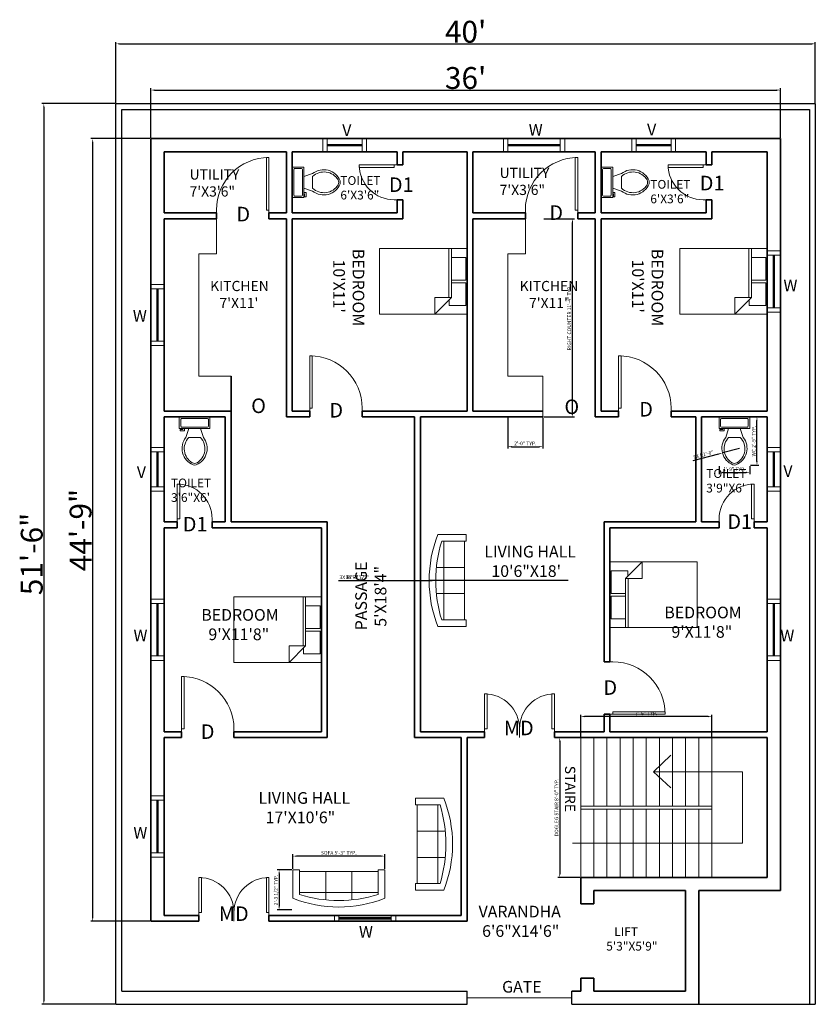
# Model space of a CAD drawing. Units: inches. Extents: x 2169 to 10664, y 1669 to 6352.
# Tile 8 of 17: x 3658 to 4204, y 1988 to 2664. Entities that reach past the tile are written whole.
import ezdxf

# ---------------------------------------------------------------- set-up
doc = ezdxf.new("R2010")
doc.units = ezdxf.units.IN
for name, color, linetype, lineweight in [('A-ANNO-DIMS', 3, 'Continuous', 18), ('A-ANNO-IDEN', 3, 'Continuous', 18), ('A-ANNO-SYMB', 6, 'Continuous', 13), ('A-AREA-IDEN', 4, 'Continuous', 18), ('A-DOOR', 4, 'Continuous', 18), ('A-FLOR-CASE', 8, 'Continuous', 18), ('A-FLOR-FIXT', 9, 'Continuous', 18), ('A-FLOR-STRS', 4, 'Continuous', 18), ('A-FURN', 8, 'Continuous', 18), ('A-GLAZ', 30, 'Continuous', 18), ('A-WALL', 7, 'Continuous', 35), ('C-PROP', 251, 'Continuous', 25)]:
    doc.layers.add(name, color=color, linetype=linetype, lineweight=lineweight)
doc.styles.get("Standard").update_dxf_attribs({"font": 'arial.ttf'})
doc.dimstyles.new('ISO-25', dxfattribs={"dimtxt": 2.5, "dimasz": 2.5, "dimexe": 1.25, "dimexo": 0.625, "dimtad": 1, "dimdec": 0, "dimlunit": 3, "dimtxsty": 'Standard', "dimcen": 2.5, "dimadec": 0, "dimazin": 0, "dimtfac": 1, "dimtdec": 0, "dimtmove": 0, "dimatfit": 3, "dimfxl": 1, "dimarcsym": 0})

# ---------------------------------------------------------------- blocks, each defined once
blk = doc.blocks.new('*U5')
for p, q in [((0, 0), (0, -6)), ((-36, 0), (-36, -6))]:
    blk.add_line(p, q)
blk.add_lwpolyline([(0, 0), (0, 36), (-1.75, 36), (-1.75, 0)], close=True)
blk.add_arc((0, 0), 36, 90, 180)
blk = doc.blocks.new('*U23')
for p, q in [((0, 0), (0, -6)), ((24, 0), (24, -6))]:
    blk.add_line(p, q)
blk.add_lwpolyline([(0, 0), (0, 24), (1.75, 24), (1.75, 0)], close=True)
blk.add_arc((0, 0), 24, 0, 90)
blk = doc.blocks.new('*U22')
for p, q in [((0, 0), (0, -6)), ((36, 0), (36, -6))]:
    blk.add_line(p, q)
blk.add_lwpolyline([(0, 0), (0, 36), (1.75, 36), (1.75, 0)], close=True)
blk.add_arc((0, 0), 36, 0, 90)
blk = doc.blocks.new('*U3')
for p, q in [((-24, 0), (-24, -6)), ((0, 0), (0, -6))]:
    blk.add_line(p, q)
blk.add_lwpolyline([(0, 0), (0, 24), (-1.75, 24), (-1.75, 0)], close=True)
blk.add_arc((0, 0), 24, 90, 180)
blk = doc.blocks.new('*U25')
for p, q in [((0, 0), (0, 6)), ((24, 0), (24, 6))]:
    blk.add_line(p, q)
blk.add_lwpolyline([(0, 0), (0, -24), (1.75, -24), (1.75, 0)], close=True)
blk.add_arc((0, 0), 24, 270, 0)
blk = doc.blocks.new('*U24')
for p, q in [((0, 0), (0, 6)), ((24, 0), (24, 6))]:
    blk.add_line(p, q)
blk.add_lwpolyline([(0, 0), (0, -24), (1.75, -24), (1.75, 0)], close=True)
blk.add_arc((0, 0), 24, 270, 0)
blk = doc.blocks.new('Bed - Queen')
for p, q in [((0, -80.00003), (0, 0)), ((0, 0), (59.99999, 0)), ((59.99999, 0), (59.99999, -80.00003)), ((7.99999, -1.2), (28.79998, -1.2)), ((7.99999, -14.4), (7.99999, -1.2)), ((28.79998, -1.2), (28.79998, -14.4)), ((31.19999, -1.2), (51.99999, -1.2)), ((31.19999, -14.4), (31.19999, -1.2)), ((51.99999, -1.2), (51.99999, -16.4)), ((0, -14.4), (44.8, -14.4)), ((44.8, -16.8), (0, -16.8)), ((59.99999, -29.6), (44.8, -14.4)), ((44.8, -14.4), (44.8, -29.6)), ((51.99999, -16.4), (46.79936, -16.4)), ((44.8, -29.6), (59.99999, -29.6)), ((59.99999, -80.00003), (0, -80.00003))]:
    blk.add_line(p, q)
blk = doc.blocks.new('Sofa - Roundback 7 ft.')
for p, q in [((-12.00002, -32.4421), (-12.00003, -6.5971)), ((11.99997, -32.4421), (11.99998, -6.5971)), ((-36.000027, -34), (-36.000027, -11.4696)), ((-35.999844, -13.3819), (35.9998, -13.3819)), ((35.99998, -34), (35.99998, -11.4696)), ((-36.000027, -32.4421), (35.99998, -32.4421))]:
    blk.add_line(p, q)
for points in [[(-36.000027, -34), (-42.000027, -34), (-42.000027, -8)], [(41.99998, -8), (41.99998, -34), (35.99998, -34)]]:
    blk.add_lwpolyline(points)
for centre, radius, start, end in [((0, -114.25), 114.25, 68.43141, 111.5686), ((-0.00001, -127.1968), 121.1968, 72.72033, 107.2797)]:
    blk.add_arc(centre, radius, start, end)
blk = doc.blocks.new('Toilet - top')
for p, q in [((9.5, -6), (9.5, -2)), ((-10, -8.5), (-8, -8.5)), ((-10, -9.5), (-10, -8.5)), ((-7, -9.5), (-10, -9.5)), ((-8, -8.5), (-8, -8)), ((-7, -8), (-7, -9.5)), ((-4, -8), (-6, -14)), ((4, -8), (6, -14)), ((4, -14), (-4, -14))]:
    blk.add_line(p, q)
blk.add_lwpolyline([(10.5, -8), (10.5, 0), (-10.5, 0), (-10.5, -8)], close=True)
for points in [[(-9.5, -2), (-9.5, -6)], [(8.5, -1), (-8.5, -1)], [(-8.5, -7), (8.5, -7)]]:
    blk.add_lwpolyline(points)
for centre, radius, start, end in [((-8.62, -1.88), 0.884, 81.8699, 188.1301), ((-8.62, -6.12), 0.884, 171.8699, 278.1301), ((8.62, -1.88), 0.884, 351.8699, 98.1301), ((8.62, -6.12), 0.884, 261.8699, 8.1301), ((3.52, -21.58), 12.17, 141.46911, 247.97143), ((4.2, -21.82), 11.33, 136.36773, 238.94682), ((-3.52, -21.58), 12.17, 292.02843, 38.53071), ((-4.2, -21.82), 11.33, 301.05301, 43.63209), ((0, -27.88), 4, 245.73182, 294.26817), ((0, -29), 4, 254.86053, 285.13947)]:
    blk.add_arc(centre, radius, start, end)
blk = doc.blocks.new('*D30')
at = {"layer": 'A-ANNO-DIMS', "color": 0, "lineweight": -2, "transparency": 16777216}
for p, q in [((3748.18, 2582.76), (3748.18, 2616.69)), ((3750.68, 2615.44), (4177.68, 2615.44)), ((4180.18, 2582.76), (4180.18, 2616.69))]:
    blk.add_line(p, q, dxfattribs=at)
at = {"layer": 'A-ANNO-DIMS', "color": 0, "transparency": 16777216}
for points in [[(3750.68, 2615.85), (3750.68, 2615.02), (3748.18, 2615.44)], [(4177.68, 2615.85), (4177.68, 2615.02), (4180.18, 2615.44)]]:
    blk.add_solid(points, dxfattribs=at)
at = {"layer": 'Defpoints', "color": 0, "transparency": 16777216}
for p in [(4180.18, 2615.44), (3748.18, 2582.13), (4180.18, 2582.13)]:
    blk.add_point(p, dxfattribs=at)
at = {"layer": 'A-ANNO-DIMS', "color": 0, "transparency": 16777216, "insert": (3964.18, 2623.72), "char_height": 2.5, "attachment_point": 5}
blk.add_mtext("{\\H6x;36'}", dxfattribs=at)
blk = doc.blocks.new('*D31')
at = {"layer": 'A-ANNO-DIMS', "color": 0, "lineweight": -2, "transparency": 16777216}
for p, q in [((3724.18, 2606.76), (3724.18, 2648.41)), ((4204.18, 2606.76), (4204.18, 2648.41)), ((3726.68, 2647.16), (4201.68, 2647.16))]:
    blk.add_line(p, q, dxfattribs=at)
at = {"layer": 'A-ANNO-DIMS', "color": 0, "transparency": 16777216}
for points in [[(3726.68, 2647.58), (3726.68, 2646.75), (3724.18, 2647.16)], [(4201.68, 2647.58), (4201.68, 2646.75), (4204.18, 2647.16)]]:
    blk.add_solid(points, dxfattribs=at)
at = {"layer": 'Defpoints', "color": 0, "transparency": 16777216}
for p in [(4204.18, 2647.16), (3724.18, 2606.13), (4204.18, 2606.13)]:
    blk.add_point(p, dxfattribs=at)
at = {"layer": 'A-ANNO-DIMS', "color": 0, "transparency": 16777216, "insert": (3964.18, 2655.45), "char_height": 2.5, "attachment_point": 5}
blk.add_mtext("{\\H6x;40'}", dxfattribs=at)
blk = doc.blocks.new('*D32')
at = {"layer": 'A-ANNO-DIMS', "color": 0, "lineweight": -2, "transparency": 16777216}
for p, q in [((3747.55, 2582.13), (3706.96, 2582.13)), ((3708.21, 2579.63), (3708.21, 2047.63)), ((3747.55, 2045.13), (3706.96, 2045.13))]:
    blk.add_line(p, q, dxfattribs=at)
at = {"layer": 'A-ANNO-DIMS', "color": 0, "transparency": 16777216}
for points in [[(3707.79, 2579.63), (3708.63, 2579.63), (3708.21, 2582.13)], [(3707.79, 2047.63), (3708.63, 2047.63), (3708.21, 2045.13)]]:
    blk.add_solid(points, dxfattribs=at)
at = {"layer": 'Defpoints', "color": 0, "transparency": 16777216}
for p in [(3748.18, 2582.13), (3708.21, 2045.13), (3748.18, 2045.13)]:
    blk.add_point(p, dxfattribs=at)
at = {"layer": 'A-ANNO-DIMS', "color": 0, "transparency": 16777216, "insert": (3699.92, 2313.54), "char_height": 2.5, "attachment_point": 5, "rotation": 90}
blk.add_mtext('{\\H6x;44\'-9"}', dxfattribs=at)
blk = doc.blocks.new('*D33')
at = {"layer": 'A-ANNO-DIMS', "color": 0, "lineweight": -2, "transparency": 16777216}
for p, q in [((3723.55, 2606.13), (3673.44, 2606.13)), ((3674.69, 2603.63), (3674.69, 1990.63)), ((3723.55, 1988.13), (3673.44, 1988.13))]:
    blk.add_line(p, q, dxfattribs=at)
at = {"layer": 'A-ANNO-DIMS', "color": 0, "transparency": 16777216}
for points in [[(3674.27, 2603.63), (3675.11, 2603.63), (3674.69, 2606.13)], [(3674.27, 1990.63), (3675.11, 1990.63), (3674.69, 1988.13)]]:
    blk.add_solid(points, dxfattribs=at)
at = {"layer": 'Defpoints', "color": 0, "transparency": 16777216}
for p in [(3724.18, 2606.13), (3674.69, 1988.13), (3724.18, 1988.13)]:
    blk.add_point(p, dxfattribs=at)
at = {"layer": 'A-ANNO-DIMS', "color": 0, "transparency": 16777216, "insert": (3666.41, 2297.13), "char_height": 2.5, "attachment_point": 5, "rotation": 90}
blk.add_mtext('{\\H6x;51\'-6"}', dxfattribs=at)
blk = doc.blocks.new('WIN-36-WALL-9')
for p, q in [((9, 42), (0, 42)), ((9, 39), (0, 39)), ((4, 39), (4, 3)), ((4.5, 39), (4.5, 3)), ((5, 39), (5, 3)), ((9, 3), (0, 3)), ((9, 0), (0, 0))]:
    blk.add_line(p, q)
blk = doc.blocks.new('WIN-24-WALL-9')
for p, q in [((9, 30), (0, 30)), ((9, 27), (0, 27)), ((4, 27), (4, 3)), ((4.5, 27), (4.5, 3)), ((5, 27), (5, 3)), ((9, 3), (0, 3)), ((9, 0), (0, 0))]:
    blk.add_line(p, q)
blk = doc.blocks.new('WIN-36-WALL-4')
for p, q in [((0, 4), (0, 0)), ((3, 4), (3, 0)), ((3, 2.5), (39, 2.5)), ((3, 2), (39, 2)), ((3, 1.5), (39, 1.5)), ((39, 4), (39, 0)), ((42, 4), (42, 0))]:
    blk.add_line(p, q)
blk = doc.blocks.new('STAIR-DOGLEG-PLAN')
for p, q in [((0, 0), (0, 96)), ((9, 49), (9, 96)), ((18, 49), (18, 96)), ((27, 49), (27, 96)), ((36, 49), (36, 96)), ((45, 49), (45, 96)), ((54, 49), (54, 96)), ((63, 49), (63, 96)), ((72, 49), (72, 96)), ((81, 49), (81, 96)), ((90, 0), (90, 96)), ((90, 49), (0, 49)), ((90, 47), (0, 47)), ((9, 0), (9, 47)), ((18, 0), (18, 47)), ((27, 0), (27, 47)), ((36, 0), (36, 47)), ((45, 0), (45, 47)), ((54, 0), (54, 47)), ((63, 0), (63, 47)), ((72, 0), (72, 47)), ((81, 0), (81, 47))]:
    blk.add_line(p, q)
blk = doc.blocks.new('STAIR-DIRECTION')
for p, q in [((55.67, 49), (67.5, 60.35)), ((116.68, 49), (55.67, 49)), ((55.67, 49), (67.5, 38.08)), ((116.68, 0), (116.68, 49)), ((0, 0), (116.68, 0))]:
    blk.add_line(p, q)
blk = doc.blocks.new('COUNTER-UTILITY-L')
for p, q in [((12, 110), (12, 84)), ((0, 0), (0, 84)), ((0, 84), (12, 84)), ((0, 0), (22, 0))]:
    blk.add_line(p, q)
blk = doc.blocks.new('COUNTER-UTILITY-R')
for p, q in [((12, 136), (12, 112)), ((0, 28), (0, 112)), ((0, 112), (12, 112)), ((0, 28), (24, 28)), ((24, 0), (24, 28))]:
    blk.add_line(p, q)
blk = doc.blocks.new('*D59')
at = {"layer": 'A-ANNO-DIMS', "color": 0, "lineweight": -2, "transparency": 16777216}
for p, q in [((4159.8, 2391.13), (4165.39, 2391.13)), ((4164.14, 2360.59), (4164.14, 2388.63)), ((4159.8, 2358.09), (4165.39, 2358.09))]:
    blk.add_line(p, q, dxfattribs=at)
at = {"layer": 'A-ANNO-DIMS', "color": 0, "transparency": 16777216}
for points in [[(4163.72, 2388.63), (4164.55, 2388.63), (4164.14, 2391.13)], [(4163.72, 2360.59), (4164.55, 2360.59), (4164.14, 2358.09)]]:
    blk.add_solid(points, dxfattribs=at)
at = {"layer": 'Defpoints', "color": 0, "transparency": 16777216}
for p in [(4159.18, 2391.13), (4164.14, 2391.13), (4159.18, 2358.09)]:
    blk.add_point(p, dxfattribs=at)
at = {"layer": 'A-ANNO-DIMS', "color": 0, "transparency": 16777216, "insert": (4162.22, 2374.61), "char_height": 2.5, "attachment_point": 5, "rotation": 90}
blk.add_mtext('WC 2\'-9" TYP.', dxfattribs=at)
blk = doc.blocks.new('*D60')
at = {"layer": 'A-ANNO-DIMS', "color": 0, "lineweight": -2, "transparency": 16777216}
for p, q in [((4138.18, 2357.46), (4138.18, 2351.88)), ((4140.68, 2353.13), (4156.68, 2353.13)), ((4159.18, 2357.46), (4159.18, 2351.88))]:
    blk.add_line(p, q, dxfattribs=at)
at = {"layer": 'A-ANNO-DIMS', "color": 0, "transparency": 16777216}
for points in [[(4140.68, 2353.55), (4140.68, 2352.71), (4138.18, 2353.13)], [(4156.68, 2353.55), (4156.68, 2352.71), (4159.18, 2353.13)]]:
    blk.add_solid(points, dxfattribs=at)
at = {"layer": 'Defpoints', "color": 0, "transparency": 16777216}
for p in [(4138.18, 2358.09), (4159.18, 2358.09), (4159.18, 2353.13)]:
    blk.add_point(p, dxfattribs=at)
at = {"layer": 'A-ANNO-DIMS', "color": 0, "transparency": 16777216, "insert": (4148.68, 2355.03), "char_height": 2.5, "attachment_point": 5}
blk.add_mtext('1\'-9" TYP.', dxfattribs=at)
blk = doc.blocks.new('*D63')
at = {"layer": 'A-ANNO-DIMS', "color": 0, "lineweight": -2, "transparency": 16777216}
for p, q in [((3845.64, 2080.98), (3845.64, 2091.06)), ((3906.14, 2089.81), (3848.14, 2089.81)), ((3908.64, 2080.98), (3908.64, 2091.06))]:
    blk.add_line(p, q, dxfattribs=at)
at = {"layer": 'A-ANNO-DIMS', "color": 0, "transparency": 16777216}
for points in [[(3848.14, 2090.22), (3848.14, 2089.39), (3845.64, 2089.81)], [(3906.14, 2090.22), (3906.14, 2089.39), (3908.64, 2089.81)]]:
    blk.add_solid(points, dxfattribs=at)
at = {"layer": 'Defpoints', "color": 0, "transparency": 16777216}
for p in [(3845.64, 2089.81), (3845.64, 2080.36), (3908.64, 2080.36)]:
    blk.add_point(p, dxfattribs=at)
at = {"layer": 'A-ANNO-DIMS', "color": 0, "transparency": 16777216, "insert": (3877.14, 2091.73), "char_height": 2.5, "attachment_point": 5}
blk.add_mtext('SOFA 5\'-3" TYP.', dxfattribs=at)
blk = doc.blocks.new('*D64')
at = {"layer": 'A-ANNO-DIMS', "color": 0, "lineweight": -2, "transparency": 16777216}
for p, q in [((3845.01, 2080.36), (3834.94, 2080.36)), ((3836.19, 2077.86), (3836.19, 2055.36)), ((3845.01, 2052.86), (3834.94, 2052.86))]:
    blk.add_line(p, q, dxfattribs=at)
at = {"layer": 'A-ANNO-DIMS', "color": 0, "transparency": 16777216}
for points in [[(3835.77, 2077.86), (3836.61, 2077.86), (3836.19, 2080.36)], [(3835.77, 2055.36), (3836.61, 2055.36), (3836.19, 2052.86)]]:
    blk.add_solid(points, dxfattribs=at)
at = {"layer": 'Defpoints', "color": 0, "transparency": 16777216}
for p in [(3845.64, 2080.36), (3836.19, 2052.86), (3845.64, 2052.86)]:
    blk.add_point(p, dxfattribs=at)
at = {"layer": 'A-ANNO-DIMS', "color": 0, "transparency": 16777216, "insert": (3834.27, 2066.61), "char_height": 2.5, "attachment_point": 5, "rotation": 90}
blk.add_mtext('2\'-3 1/2" TYP.', dxfattribs=at)
blk = doc.blocks.new('*D77')
at = {"layer": 'A-ANNO-DIMS', "color": 0, "lineweight": -2, "transparency": 16777216}
for p, q in [((4042.55, 2171.13), (4027.53, 2171.13)), ((4028.78, 2168.63), (4028.78, 2077.63)), ((4042.55, 2075.13), (4027.53, 2075.13))]:
    blk.add_line(p, q, dxfattribs=at)
at = {"layer": 'A-ANNO-DIMS', "color": 0, "transparency": 16777216}
for points in [[(4028.36, 2168.63), (4029.2, 2168.63), (4028.78, 2171.13)], [(4028.36, 2077.63), (4029.2, 2077.63), (4028.78, 2075.13)]]:
    blk.add_solid(points, dxfattribs=at)
at = {"layer": 'Defpoints', "color": 0, "transparency": 16777216}
for p in [(4043.18, 2171.13), (4028.78, 2075.13), (4043.18, 2075.13)]:
    blk.add_point(p, dxfattribs=at)
at = {"layer": 'A-ANNO-DIMS', "color": 0, "transparency": 16777216, "insert": (4026.86, 2123.13), "char_height": 2.5, "attachment_point": 5, "rotation": 90}
blk.add_mtext('DOGLEG STAIR 8\'-0" TYP.', dxfattribs=at)
blk = doc.blocks.new('*D78')
at = {"layer": 'A-ANNO-DIMS', "color": 0, "lineweight": -2, "transparency": 16777216}
for p, q in [((4043.18, 2171.76), (4043.18, 2186.78)), ((4130.68, 2185.53), (4045.68, 2185.53)), ((4133.18, 2171.76), (4133.18, 2186.78))]:
    blk.add_line(p, q, dxfattribs=at)
at = {"layer": 'A-ANNO-DIMS', "color": 0, "transparency": 16777216}
for points in [[(4045.68, 2185.95), (4045.68, 2185.12), (4043.18, 2185.53)], [(4130.68, 2185.95), (4130.68, 2185.12), (4133.18, 2185.53)]]:
    blk.add_solid(points, dxfattribs=at)
at = {"layer": 'Defpoints', "color": 0, "transparency": 16777216}
for p in [(4043.18, 2185.53), (4043.18, 2171.13), (4133.18, 2171.13)]:
    blk.add_point(p, dxfattribs=at)
at = {"layer": 'A-ANNO-DIMS', "color": 0, "transparency": 16777216, "insert": (4088.18, 2187.44), "char_height": 2.5, "attachment_point": 5}
blk.add_mtext('7\'-6" TYP.', dxfattribs=at)
blk = doc.blocks.new('*D83')
at = {"layer": 'A-ANNO-DIMS', "color": 0, "lineweight": -2, "transparency": 16777216}
for p, q in [((4017.8, 2527.13), (4038.83, 2527.13)), ((4037.58, 2393.63), (4037.58, 2524.63)), ((4017.8, 2391.13), (4038.83, 2391.13))]:
    blk.add_line(p, q, dxfattribs=at)
at = {"layer": 'A-ANNO-DIMS', "color": 0, "transparency": 16777216}
for points in [[(4037.16, 2524.63), (4038, 2524.63), (4037.58, 2527.13)], [(4037.16, 2393.63), (4038, 2393.63), (4037.58, 2391.13)]]:
    blk.add_solid(points, dxfattribs=at)
at = {"layer": 'Defpoints', "color": 0, "transparency": 16777216}
for p in [(4017.18, 2527.13), (4037.58, 2527.13), (4017.18, 2391.13)]:
    blk.add_point(p, dxfattribs=at)
at = {"layer": 'A-ANNO-DIMS', "color": 0, "transparency": 16777216, "insert": (4035.66, 2459.13), "char_height": 2.5, "attachment_point": 5, "rotation": 90}
blk.add_mtext('RIGHT COUNTER 11\'-4" TYP.', dxfattribs=at)
blk = doc.blocks.new('*D84')
at = {"layer": 'A-ANNO-DIMS', "color": 0, "lineweight": -2, "transparency": 16777216}
for p, q in [((3993.18, 2390.51), (3993.18, 2369.48)), ((4017.18, 2390.51), (4017.18, 2369.48)), ((3995.68, 2370.73), (4014.68, 2370.73))]:
    blk.add_line(p, q, dxfattribs=at)
at = {"layer": 'A-ANNO-DIMS', "color": 0, "transparency": 16777216}
for points in [[(3995.68, 2371.15), (3995.68, 2370.32), (3993.18, 2370.73)], [(4014.68, 2371.15), (4014.68, 2370.32), (4017.18, 2370.73)]]:
    blk.add_solid(points, dxfattribs=at)
at = {"layer": 'Defpoints', "color": 0, "transparency": 16777216}
for p in [(3993.18, 2391.13), (4017.18, 2391.13), (4017.18, 2370.73)]:
    blk.add_point(p, dxfattribs=at)
at = {"layer": 'A-ANNO-DIMS', "color": 0, "transparency": 16777216, "insert": (4005.18, 2372.64), "char_height": 2.5, "attachment_point": 5}
blk.add_mtext('2\'-0" TYP.', dxfattribs=at)
blk = doc.blocks.new('*D135')
at = {"layer": 'A-ANNO-DIMS', "color": 0, "lineweight": -2, "transparency": 16777216}
for p, q in [((3881.27, 2278.91), (3941.14, 2278.91)), ((4034.54, 2278.91), (3943.64, 2278.91))]:
    blk.add_line(p, q, dxfattribs=at)
at = {"layer": 'A-ANNO-DIMS', "color": 0, "transparency": 16777216}
blk.add_solid([(3941.14, 2279.33), (3941.14, 2278.5), (3943.64, 2278.91)], dxfattribs=at)
at = {"layer": 'Defpoints', "color": 0, "transparency": 16777216}
for p in [(3943.64, 2278.91), (4034.54, 2278.91)]:
    blk.add_point(p, dxfattribs=at)
at = {"layer": 'A-ANNO-DIMS', "color": 0, "transparency": 16777216, "insert": (3889.1, 2280.82), "char_height": 2.5, "attachment_point": 5}
blk.add_mtext('3X R7\'-7"', dxfattribs=at)
blk = doc.blocks.new('*D136')
at = {"layer": 'A-ANNO-DIMS', "color": 0, "lineweight": -2, "transparency": 16777216}
for p, q in [((3876.99, 2278.91), (3936.64, 2278.91)), ((4024.83, 2278.91), (3939.14, 2278.91))]:
    blk.add_line(p, q, dxfattribs=at)
at = {"layer": 'A-ANNO-DIMS', "color": 0, "transparency": 16777216}
blk.add_solid([(3936.64, 2279.33), (3936.64, 2278.5), (3939.14, 2278.91)], dxfattribs=at)
at = {"layer": 'Defpoints', "color": 0, "transparency": 16777216}
for p in [(3939.14, 2278.91), (4024.83, 2278.91)]:
    blk.add_point(p, dxfattribs=at)
at = {"layer": 'A-ANNO-DIMS', "color": 0, "transparency": 16777216, "insert": (3887.73, 2280.83), "char_height": 2.5, "attachment_point": 5}
blk.add_mtext('3X R7\'-1 1/2"', dxfattribs=at)
blk = doc.blocks.new('*D137')
at = {"layer": 'A-ANNO-DIMS', "color": 0, "lineweight": -2, "transparency": 16777216}
for p, q in [((4120.44, 2361.21), (4138.01, 2365.83)), ((4152.2, 2369.55), (4140.43, 2366.46))]:
    blk.add_line(p, q, dxfattribs=at)
at = {"layer": 'A-ANNO-DIMS', "color": 0, "transparency": 16777216}
blk.add_solid([(4137.9, 2366.23), (4138.12, 2365.42), (4140.43, 2366.46)], dxfattribs=at)
at = {"layer": 'Defpoints', "color": 0, "transparency": 16777216}
for p in [(4140.43, 2366.46), (4152.2, 2369.55)]:
    blk.add_point(p, dxfattribs=at)
at = {"layer": 'A-ANNO-DIMS', "color": 0, "transparency": 16777216, "insert": (4127.53, 2365.04), "char_height": 2.5, "attachment_point": 5, "rotation": 14.71856}
blk.add_mtext('8X R1\'-0"', dxfattribs=at)

msp = doc.modelspace()

# ---------------------------------------------------------------- linework, layer by layer
at = {"layer": 'A-DOOR'}
msp.add_line((3965.18, 1992.63), (4037.18, 1992.63), dxfattribs=at)
at = {"layer": 'A-WALL'}
for p, q in [((3748.18, 2582.13), (4180.18, 2582.13)), ((3748.18, 2045.13), (3748.18, 2582.13)), ((4180.18, 2582.13), (4180.18, 2066.13)), ((3757.18, 2573.13), (3841.18, 2573.13)), ((3757.18, 2531.13), (3757.18, 2573.13)), ((3841.18, 2531.13), (3841.18, 2573.13)), ((3845.18, 2573.13), (3917.18, 2573.13)), ((3845.18, 2531.13), (3845.18, 2573.13)), ((3917.18, 2564.13), (3917.18, 2573.13)), ((3921.18, 2573.13), (3965.18, 2573.13)), ((3921.18, 2564.13), (3921.18, 2573.13)), ((3965.18, 2395.13), (3965.18, 2573.13)), ((3969.18, 2573.13), (4053.18, 2573.13)), ((3969.18, 2531.13), (3969.18, 2573.13)), ((4053.18, 2531.13), (4053.18, 2573.13)), ((4057.18, 2573.13), (4129.18, 2573.13)), ((4057.18, 2531.13), (4057.18, 2573.13)), ((4129.18, 2564.13), (4129.18, 2573.13)), ((4133.18, 2573.13), (4171.18, 2573.13)), ((4133.18, 2564.13), (4133.18, 2573.13)), ((4171.18, 2573.13), (4171.18, 2395.13)), ((3917.18, 2564.13), (3921.18, 2564.13)), ((4129.18, 2564.13), (4133.18, 2564.13)), ((3917.18, 2531.13), (3917.18, 2540.13)), ((3917.18, 2540.13), (3921.18, 2540.13)), ((3921.18, 2527.13), (3921.18, 2540.13)), ((4129.18, 2531.13), (4129.18, 2540.13)), ((4129.18, 2540.13), (4133.18, 2540.13)), ((4133.18, 2527.13), (4133.18, 2540.13)), ((3757.18, 2531.13), (3793.18, 2531.13)), ((3757.18, 2527.13), (3793.18, 2527.13)), ((3757.18, 2395.13), (3757.18, 2527.13)), ((3793.18, 2527.13), (3793.18, 2531.13)), ((3829.18, 2531.13), (3841.18, 2531.13)), ((3829.18, 2527.13), (3829.18, 2531.13)), ((3829.18, 2527.13), (3841.18, 2527.13)), ((3841.18, 2391.13), (3841.18, 2527.13)), ((3845.18, 2531.13), (3917.18, 2531.13)), ((3845.18, 2527.13), (3921.18, 2527.13)), ((3845.18, 2395.13), (3845.18, 2527.13)), ((3969.18, 2531.13), (4005.18, 2531.13)), ((3969.18, 2527.13), (4005.18, 2527.13)), ((3969.18, 2395.13), (3969.18, 2527.13)), ((4005.18, 2527.13), (4005.18, 2531.13)), ((4041.18, 2531.13), (4053.18, 2531.13)), ((4041.18, 2527.13), (4041.18, 2531.13)), ((4041.18, 2527.13), (4053.18, 2527.13)), ((4053.18, 2391.13), (4053.18, 2527.13)), ((4057.18, 2531.13), (4129.18, 2531.13)), ((4057.18, 2527.13), (4133.18, 2527.13)), ((4057.18, 2395.13), (4057.18, 2527.13)), ((3803.18, 2319.13), (3803.18, 2419.13)), ((3757.18, 2395.13), (3803.18, 2395.13)), ((3845.18, 2395.13), (3857.18, 2395.13)), ((3857.18, 2391.13), (3857.18, 2395.13)), ((3893.18, 2395.13), (3965.18, 2395.13)), ((3893.18, 2391.13), (3893.18, 2395.13)), ((3969.18, 2395.13), (4017.18, 2395.13)), ((4057.18, 2395.13), (4069.18, 2395.13)), ((4069.18, 2391.13), (4069.18, 2395.13)), ((4105.18, 2395.13), (4171.18, 2395.13)), ((4105.18, 2391.13), (4105.18, 2395.13)), ((3757.18, 2391.13), (3799.18, 2391.13)), ((3757.18, 2319.13), (3757.18, 2391.13)), ((3799.18, 2319.13), (3799.18, 2391.13)), ((3841.18, 2391.13), (3857.18, 2391.13)), ((3893.18, 2391.13), (3929.18, 2391.13)), ((3929.18, 2171.13), (3929.18, 2391.13)), ((3933.18, 2391.13), (4017.18, 2391.13)), ((3933.18, 2175.13), (3933.18, 2391.13)), ((4053.18, 2391.13), (4069.18, 2391.13)), ((4105.18, 2391.13), (4122.18, 2391.13)), ((4122.18, 2391.13), (4122.18, 2319.13)), ((4126.18, 2391.13), (4171.18, 2391.13)), ((4126.18, 2391.13), (4126.18, 2319.13)), ((4171.18, 2391.13), (4171.18, 2319.13)), ((3757.18, 2319.13), (3766.18, 2319.13)), ((3766.18, 2315.13), (3766.18, 2319.13)), ((3790.18, 2319.13), (3799.18, 2319.13)), ((3790.18, 2315.13), (3790.18, 2319.13)), ((3803.18, 2319.13), (3869.18, 2319.13)), ((3869.18, 2171.13), (3869.18, 2319.13)), ((4059.18, 2319.13), (4122.18, 2319.13)), ((4059.18, 2319.13), (4059.18, 2223.13)), ((4126.18, 2319.13), (4138.18, 2319.13)), ((4138.18, 2319.13), (4138.18, 2315.13)), ((4162.18, 2319.13), (4171.18, 2319.13)), ((4162.18, 2319.13), (4162.18, 2315.13)), ((3757.18, 2315.13), (3766.18, 2315.13)), ((3757.18, 2175.13), (3757.18, 2315.13)), ((3790.18, 2315.13), (3865.18, 2315.13)), ((3865.18, 2175.13), (3865.18, 2315.13)), ((4063.18, 2315.13), (4138.18, 2315.13)), ((4063.18, 2315.13), (4063.18, 2223.13)), ((4162.18, 2315.13), (4171.18, 2315.13)), ((4171.18, 2315.13), (4171.18, 2175.13)), ((4059.18, 2223.13), (4063.18, 2223.13)), ((4059.18, 2187.13), (4063.18, 2187.13)), ((4059.18, 2187.13), (4059.18, 2175.13)), ((4063.18, 2187.13), (4063.18, 2175.13)), ((3757.18, 2175.13), (3769.18, 2175.13)), ((3757.18, 2171.13), (3769.18, 2171.13)), ((3757.18, 2049.13), (3757.18, 2171.13)), ((3769.18, 2171.13), (3769.18, 2175.13)), ((3805.18, 2175.13), (3865.18, 2175.13)), ((3805.18, 2171.13), (3805.18, 2175.13)), ((3805.18, 2171.13), (3869.18, 2171.13)), ((3929.18, 2171.13), (3961.18, 2171.13)), ((3933.18, 2175.13), (3977.18, 2175.13)), ((3961.18, 2049.13), (3961.18, 2171.13)), ((3965.18, 2171.13), (3977.18, 2171.13)), ((3965.18, 2045.13), (3965.18, 2171.13)), ((3977.18, 2171.13), (3977.18, 2175.13)), ((4025.18, 2175.13), (4059.18, 2175.13)), ((4025.18, 2171.13), (4025.18, 2175.13)), ((4025.18, 2171.13), (4171.18, 2171.13)), ((4063.18, 2175.13), (4171.18, 2175.13)), ((4171.18, 2171.13), (4171.18, 2075.13)), ((4171.18, 2075.13), (4043.18, 2075.13)), ((4043.18, 2057.13), (4043.18, 2075.13)), ((4115.18, 2066.13), (4052.18, 2066.13)), ((4052.18, 2057.13), (4052.18, 2066.13)), ((4115.18, 1997.13), (4115.18, 2066.13)), ((4180.18, 2066.13), (4124.18, 2066.13)), ((4124.18, 1988.13), (4124.18, 2066.13)), ((4052.18, 2057.13), (4043.18, 2057.13)), ((3781.18, 2049.13), (3757.18, 2049.13)), ((3781.18, 2045.13), (3781.18, 2049.13)), ((3961.18, 2049.13), (3829.18, 2049.13)), ((3829.18, 2045.13), (3829.18, 2049.13)), ((3781.18, 2045.13), (3748.18, 2045.13)), ((3965.18, 2045.13), (3829.18, 2045.13)), ((4043.18, 1997.13), (4043.18, 2006.13)), ((4043.18, 2006.13), (4052.18, 2006.13)), ((4052.18, 1997.13), (4052.18, 2006.13)), ((4037.18, 1997.13), (4043.18, 1997.13)), ((4052.18, 1997.13), (4115.18, 1997.13))]:
    msp.add_line(p, q, dxfattribs=at)
at = {"layer": 'C-PROP'}
for p, q in [((3724.18, 2606.13), (4204.18, 2606.13)), ((3724.18, 1988.13), (3724.18, 2606.13)), ((3728.18, 2602.13), (4200.18, 2602.13)), ((3728.18, 1997.13), (3728.18, 2602.13)), ((4200.18, 2602.13), (4200.18, 1988.13)), ((4204.18, 2606.13), (4204.18, 1988.13)), ((3728.18, 1997.13), (3965.18, 1997.13)), ((3965.18, 1988.13), (3965.18, 1997.13)), ((4037.18, 1988.13), (4037.18, 1997.13)), ((3724.18, 1988.13), (3965.18, 1988.13)), ((4037.18, 1988.13), (4124.18, 1988.13)), ((4124.18, 1988.13), (4204.18, 1988.13))]:
    msp.add_line(p, q, dxfattribs=at)

# ---------------------------------------------------------------- block references
at = {"layer": 'A-ANNO-SYMB'}
msp.add_blockref('STAIR-DIRECTION', (4037.5, 2098.63), dxfattribs=at)
at = {"layer": 'A-DOOR'}
for name, p in [('*U5', (3829.18, 2533.13)), ('*U5', (4041.18, 2533.13)), ('*U22', (3857.18, 2397.13)), ('*U22', (4069.18, 2397.13)), ('*U23', (3766.18, 2321.13)), ('*U3', (4162.18, 2321.13)), ('*U22', (3769.18, 2177.13)), ('*U23', (3977.18, 2177.13)), ('*U3', (4025.18, 2177.13)), ('*U23', (3781.18, 2051.13)), ('*U3', (3829.18, 2051.13))]:
    msp.add_blockref(name, p, dxfattribs=at)
at = {"layer": 'A-DOOR', "rotation": 270}
for name, p in [('*U24', (3915.18, 2564.13)), ('*U25', (4127.18, 2564.13)), ('*U5', (4065.18, 2187.13))]:
    msp.add_blockref(name, p, dxfattribs=at)
at = {"layer": 'A-FLOR-CASE'}
for name, p in [('COUNTER-UTILITY-L', (3781.18, 2419.13)), ('COUNTER-UTILITY-R', (3993.18, 2391.13))]:
    msp.add_blockref(name, p, dxfattribs=at)
at = {"layer": 'A-FLOR-FIXT', "rotation": 90}
for p in [(3845.18, 2552.13), (4057.18, 2552.13)]:
    msp.add_blockref('Toilet - top', p, dxfattribs=at)
at = {"layer": 'A-FLOR-FIXT'}
for p in [(3778.18, 2391.13), (4148.68, 2391.13)]:
    msp.add_blockref('Toilet - top', p, dxfattribs=at)
at = {"layer": 'A-FLOR-STRS', "rotation": 180}
msp.add_blockref('STAIR-DOGLEG-PLAN', (4133.18, 2171.13), dxfattribs=at)
at = {"layer": 'A-FURN', "xscale": 0.75, "yscale": 0.75, "zscale": 0.75}
for name, p, rotation in [('Bed - Queen', (3965.18, 2506.63), 270), ('Bed - Queen', (4171.18, 2506.63), 270), ('Sofa - Roundback 7 ft.', (3939.14, 2278.91), 89.99999999999999), ('Bed - Queen', (4063.18, 2246.63), 89.99999999999999), ('Bed - Queen', (3865.18, 2267.63), 270), ('Sofa - Roundback 7 ft.', (3955.21, 2097.98), 270), ('Sofa - Roundback 7 ft.', (3877.14, 2054.86), 180)]:
    msp.add_blockref(name, p, dxfattribs=dict(at, rotation=rotation))
at = {"layer": 'A-GLAZ'}
for name, p, rotation in [('WIN-24-WALL-9', (3866.18, 2582.13), 270.0000000000009), ('WIN-36-WALL-9', (4032.18, 2573.13), 89.99999999999804), ('WIN-24-WALL-9', (4078.18, 2582.13), 269.9999999999978), ('WIN-36-WALL-9', (4180.18, 2505.13), 180), ('WIN-36-WALL-9', (3757.18, 2482.13), 180), ('WIN-36-WALL-9', (3757.18, 2266.13), 180), ('WIN-36-WALL-9', (4180.18, 2266.13), 180), ('WIN-36-WALL-9', (3757.18, 2131.13), 180), ('WIN-36-WALL-4', (3916.18, 2049.13), 180)]:
    msp.add_blockref(name, p, dxfattribs=dict(at, rotation=rotation))
for p in [(3748.18, 2340.13), (4171.18, 2340.13)]:
    msp.add_blockref('WIN-24-WALL-9', p, dxfattribs=at)

# ---------------------------------------------------------------- texts
at = {"layer": 'A-ANNO-IDEN', "attachment_point": 1}
for s, heights, insert, char_height in [('V', [8.65], (3879.49, 2591.95), 8), ('W', [8.65], (4007.49, 2592.17), 8), ('V', [8.65], (4088.72, 2592.29), 8), ('D1', [0], (3911.54, 2555.51), 10), ('D1', [0], (4124.88, 2556.61), 10), ('D', [0], (3806.88, 2535.32), 10), ('D', [0], (4021.65, 2536.37), 10), ('W', [8.65], (4182.31, 2485.36), 8), ('W', [8.65], (3735.8, 2464.43), 8), ('O', [8.65], (3817.01, 2403.81), 10), ('D', [0], (3870.68, 2400.76), 10), ('O', [8.65], (4031.99, 2403.12), 10), ('D', [0], (4083.35, 2401.43), 10), ('V', [8.65], (4182.25, 2357.98), 8), ('V', [8.65], (3738.53, 2357.31), 8), ('D1', [0], (4143.84, 2324.31), 10), ('D1', [0], (3770.06, 2322.56), 10), ('W', [8.65], (3736.24, 2245.27), 8), ('W', [8.65], (4180.18, 2245.09), 8), ('D', [0], (4058.78, 2210.45), 10), ('MD', [8.65], (3990.44, 2182.72), 10), ('D', [0], (3782.43, 2180.23), 10), ('W', [8.65], (3736.15, 2109.9), 8), ('MD', [8.65], (3794.83, 2055.31), 10), ('W', [8.65], (3890.98, 2041.8), 8)]:
    msp.add_mtext_dynamic_manual_height_columns(s, width=418.9353, gutter_width=12.5, heights=heights, dxfattribs=dict(at, insert=insert, char_height=char_height))
at = {"layer": 'A-AREA-IDEN', "attachment_point": 1}
for s, width, insert, char_height in [('UTILITY\\P7\'X3\'6"', 378.2909, (3774.72, 2561.04), 7), ('UTILITY\\P7\'X3\'6"', 378.2909, (3987.5, 2562.11), 7), ('TOILET\\P6\'X3\'6"', 229.0681, (3878.21, 2556.38), 6), ('TOILET\\P6\'X3\'6"', 229.0681, (4090.94, 2553.76), 6), ("KITCHEN\\P   7'X11'", 624.2169, (3788.83, 2484.5), 7), ("KITCHEN\\P   7'X11'", 624.2169, (4001.28, 2484.46), 7), ('TOILET\\P3\'9"X6\'', 181.098, (4129.33, 2355.33), 6), ('TOILET\\P3\'6"X6\'', 181.098, (3762, 2348.85), 6), ('LIVING HALL\\P  10\'6"X18\'', 560.0068, (3977, 2302.72), 8), ('BEDROOM\\P  9\'X11\'8"', 585.4842, (3782.77, 2259.33), 8), ('BEDROOM\\P  9\'X11\'8"', 585.4842, (4100.57, 2260.98), 8), ('LIVING HALL\\P  17\'X10\'6"', 430.6105, (3822.01, 2133.71), 8), ('VARANDHA\\P 6\'6"X14\'6"', 244.2229, (3973.08, 2055.75), 8), ('   LIFT\\P5\'3"X5\'9"', 367.579, (4060.69, 2041.01), 6), ('GATE', 121.9604, (3989.22, 2004.15), 8)]:
    msp.add_mtext_dynamic_manual_height_columns(s, width=width, gutter_width=12.5, heights=[0], dxfattribs=dict(at, insert=insert, char_height=char_height))
for s, width, insert, char_height, rotation in [("BEDROOM\\P   10'X11'", 613.8035, (3894.65, 2506.49), 8, 270), ("BEDROOM\\P   10'X11'", 613.8035, (4099.78, 2506.49), 8, 270), ('PASSAGE\\P 5\'X18\'4"', 733.7273, (3888.46, 2244.77), 8, 90), ('STAIRE', 319.0814, (4039.42, 2151.81), 7, 270)]:
    msp.add_mtext_dynamic_manual_height_columns(s, width=width, gutter_width=12.5, heights=[0], dxfattribs=dict(at, insert=insert, char_height=char_height, rotation=rotation))

# ---------------------------------------------------------------- dimensions: what is measured, and where the dimension line sits
at = {"layer": 'A-ANNO-DIMS'}
for base, p1, p2, text, override, picture, middle in [((4204.18, 2647.16), (3724.18, 2606.13), (4204.18, 2606.13), '{\\H6x;<>}', {"dimclrd": 0, "dimclre": 0, "dimclrt": 0}, '*D31', (3964.18, 2655.45)), ((4017.18, 2370.73), (3993.18, 2391.13), (4017.18, 2391.13), '<> TYP.', {"dimdec": 1, "dimlfac": 1, "dimrnd": 0, "dimzin": 1, "dimdsep": 46, "dimlunit": 4, "dimfrac": 2}, '*D84', (4005.18, 2372.64)), ((4159.18, 2353.13), (4138.18, 2358.09), (4159.18, 2358.09), '<> TYP.', {"dimdec": 1, "dimlfac": 1, "dimrnd": 0, "dimzin": 1, "dimdsep": 46, "dimlunit": 4, "dimfrac": 2}, '*D60', (4148.68, 2355.03))]:
    dim = msp.add_linear_dim(base=base, p1=p1, p2=p2, text=text, dimstyle='ISO-25', override=override, dxfattribs=at)
    dim.commit()
    dim.dimension.update_dxf_attribs({"geometry": picture, "text_midpoint": middle})
dim = msp.add_linear_dim(base=(4180.18, 2615.44), p1=(3748.18, 2582.13), p2=(4180.18, 2582.13), text='{\\H6x;<>}', dimstyle='ISO-25', override={"dimclrd": 0, "dimclre": 0, "dimclrt": 0}, dxfattribs=at)
dim.commit()
dim.dimension.update_dxf_attribs({"geometry": '*D30', "text_midpoint": (3964.18, 2615.44), "dimtype": 160})
for base, p1, p2, picture, middle in [((3674.69, 1988.13), (3724.18, 2606.13), (3724.18, 1988.13), '*D33', (3674.69, 2297.13)), ((3708.21, 2045.13), (3748.18, 2582.13), (3748.18, 2045.13), '*D32', (3708.21, 2313.54))]:
    dim = msp.add_linear_dim(base=base, p1=p1, p2=p2, angle=90, text='{\\H6x;<>}', dimstyle='ISO-25', override={"dimclrd": 0, "dimclre": 0, "dimclrt": 0}, dxfattribs=at)
    dim.commit()
    dim.dimension.update_dxf_attribs({"geometry": picture, "text_midpoint": middle, "dimtype": 160})
for base, p1, p2, angle, text, picture, middle in [((4037.58, 2527.13), (4017.18, 2391.13), (4017.18, 2527.13), 90, 'RIGHT COUNTER <> TYP.', '*D83', (4035.66, 2459.13)), ((4164.14, 2391.13), (4159.18, 2358.09), (4159.18, 2391.13), 90, 'WC <> TYP.', '*D59', (4162.22, 2374.61)), ((4043.18, 2185.53), (4133.18, 2171.13), (4043.18, 2171.13), 180, '<> TYP.', '*D78', (4088.18, 2187.44)), ((4028.78, 2075.13), (4043.18, 2171.13), (4043.18, 2075.13), 270, 'DOGLEG STAIR <> TYP.', '*D77', (4026.86, 2123.13)), ((3845.64, 2089.81), (3908.64, 2080.36), (3845.64, 2080.36), 180, 'SOFA <> TYP.', '*D63', (3877.14, 2091.73)), ((3836.19, 2052.86), (3845.64, 2080.36), (3845.64, 2052.86), 270, '<> TYP.', '*D64', (3834.27, 2066.61))]:
    dim = msp.add_linear_dim(base=base, p1=p1, p2=p2, angle=angle, text=text, dimstyle='ISO-25', override={"dimdec": 1, "dimlfac": 1, "dimrnd": 0, "dimzin": 1, "dimdsep": 46, "dimlunit": 4, "dimfrac": 2}, dxfattribs=at)
    dim.commit()
    dim.dimension.update_dxf_attribs({"geometry": picture, "text_midpoint": middle})
dim = msp.add_radius_dim(center=(4152.2, 2369.55), mpoint=(4140.43, 2366.46), text='8X <>', dimstyle='ISO-25', override={"dimdec": 1, "dimlfac": 1, "dimrnd": 0, "dimzin": 1, "dimdsep": 46, "dimlunit": 4, "dimfrac": 2}, dxfattribs=at)
dim.commit()
dim.dimension.update_dxf_attribs({"geometry": '*D137', "text_midpoint": (4127.53, 2365.04)})
for center, mpoint, picture, middle in [((4024.83, 2278.91), (3939.14, 2278.91), '*D136', (3887.73, 2278.91)), ((4034.54, 2278.91), (3943.64, 2278.91), '*D135', (3889.1, 2278.91))]:
    dim = msp.add_radius_dim(center=center, mpoint=mpoint, text='3X <>', dimstyle='ISO-25', override={"dimdec": 1, "dimlfac": 1, "dimrnd": 0, "dimzin": 1, "dimdsep": 46, "dimlunit": 4, "dimfrac": 2}, dxfattribs=at)
    dim.commit()
    dim.dimension.update_dxf_attribs({"geometry": picture, "text_midpoint": middle, "dimtype": 164})

doc.saveas('drawing.dxf')
